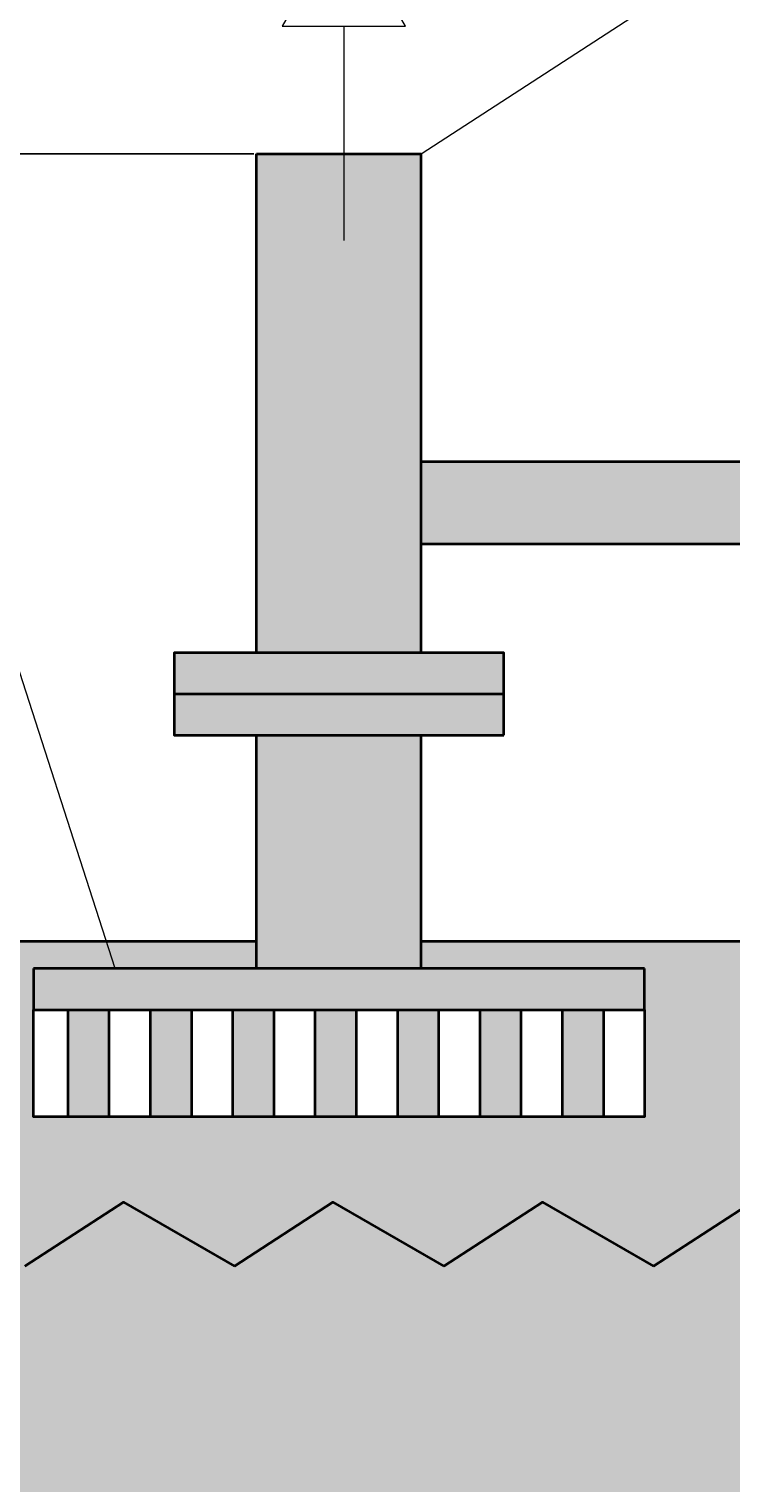
# Model space of a CAD drawing. Units: inches. Extents: x -1 to 292, y -3 to 199.
# Tile 28 of 52: x 106 to 123, y 95 to 130. Entities that reach past the tile are written whole.
import ezdxf

# ---------------------------------------------------------------- set-up
doc = ezdxf.new("R2010")
doc.units = ezdxf.units.IN
doc.header["$MEASUREMENT"] = 0
for name, color, linetype, lineweight in [('M-ANNO-LEAD', 2, 'Continuous', 18), ('M-ANNO-SYMB', 1, 'Continuous', 18), ('M-DIMS', 2, 'Continuous', 18), ('M-EQPM', 7, 'Continuous', 35), ('M-PATT', 8, 'Continuous', 13)]:
    doc.layers.add(name, color=color, linetype=linetype, lineweight=lineweight)
doc.styles.get("Standard").update_dxf_attribs({"font": 'arial.ttf'})
doc.dimstyles.get("Standard").update_dxf_attribs({"dimtxt": 0.18, "dimasz": 0.18, "dimexe": 0.18, "dimexo": 0.0625, "dimgap": 0.09, "dimtad": 0, "dimtih": 1, "dimtoh": 1, "dimdec": 4, "dimzin": 0, "dimdsep": 46, "dimtxsty": 'Standard', "dimcen": 0.09, "dimadec": 0, "dimazin": 0, "dimtfac": 1, "dimtdec": 4, "dimtofl": 0, "dimtmove": 0, "dimatfit": 3, "dimfxl": 1, "dimtolj": 1, "dimtzin": 0, "dimarcsym": 0})

# ---------------------------------------------------------------- blocks, each defined once
blk = doc.blocks.new('ARROW-STEAM-OUT')
blk.add_line((113.608, 129.862), (113.608, 124.666))
blk.add_lwpolyline([(112.108, 129.862), (115.108, 129.862), (113.608, 132.46)], close=True)
blk = doc.blocks.new('*D8')
at = {"layer": 'Defpoints', "color": 0, "transparency": 16777216}
for p in [(-0.662, 126.765), (111.488, 126.765), (69.013, 25.514)]:
    blk.add_point(p, dxfattribs=at)
at = {"layer": 'M-DIMS', "color": 0, "lineweight": -2, "transparency": 16777216}
for p, q in [((111.426, 126.765), (-0.842, 126.765)), ((-0.662, 126.585), (-0.662, 76.321)), ((-0.662, 25.694), (-0.662, 75.958)), ((68.951, 25.514), (-0.842, 25.514))]:
    blk.add_line(p, q, dxfattribs=at)
at = {"layer": 'M-DIMS', "color": 0, "transparency": 16777216}
for points in [[(-0.692, 126.585), (-0.632, 126.585), (-0.662, 126.765)], [(-0.692, 25.694), (-0.632, 25.694), (-0.662, 25.514)]]:
    blk.add_solid(points, dxfattribs=at)
at = {"layer": 'M-DIMS', "color": 0, "transparency": 16777216, "insert": (-0.662, 76.14), "char_height": 0.18, "attachment_point": 5}
blk.add_mtext('\\A1;101.25', dxfattribs=at)
blk = doc.blocks.new('*D9')
at = {"layer": 'Defpoints', "color": 0, "transparency": 16777216}
for p in [(177.053, 174.363), (49.924, 99.774), (177.053, 99.774)]:
    blk.add_point(p, dxfattribs=at)
at = {"layer": 'M-DIMS', "color": 0, "lineweight": -2, "transparency": 16777216}
for p, q in [((49.924, 99.836), (49.924, 174.543)), ((50.104, 174.363), (113.033, 174.363)), ((176.873, 174.363), (113.943, 174.363)), ((177.053, 99.836), (177.053, 174.543))]:
    blk.add_line(p, q, dxfattribs=at)
at = {"layer": 'M-DIMS', "color": 0, "transparency": 16777216}
for points in [[(50.104, 174.393), (50.104, 174.333), (49.924, 174.363)], [(176.873, 174.393), (176.873, 174.333), (177.053, 174.363)]]:
    blk.add_solid(points, dxfattribs=at)
at = {"layer": 'M-DIMS', "color": 0, "transparency": 16777216, "insert": (113.488, 174.363), "char_height": 0.18, "attachment_point": 5}
blk.add_mtext('\\A1;127.13', dxfattribs=at)

msp = doc.modelspace()

# ---------------------------------------------------------------- hatches: boundary and pattern name
at = {"layer": 'M-PATT'}
h = msp.add_hatch(color=256, dxfattribs=at)
h.set_gradient(color1=(0, 127, 0), color2=(0, 127, 0), tint=1, name='CYLINDER')
h.paths.add_polyline_path([(164.5186, 119.2985), (129.9293, 119.2985), (129.9293, 117.2985), (164.1897, 117.2985)])
h.paths.add_polyline_path([(181.5897, 119.2985), (164.5186, 119.2985), (164.1897, 117.2985), (179.5897, 117.2985), (179.5897, 107.8518), (181.5897, 109.1506)])
h.paths.add_polyline_path([(181.5897, 109.1506), (179.5897, 107.8518), (179.5897, 36.2698), (198.4159, 36.2698), (198.4159, 38.2698), (181.5897, 38.2698)])
h.paths.add_polyline_path([(115.4883, 126.765), (111.4883, 126.765), (111.4883, 114.6589), (115.4883, 114.6589)])
h.paths.add_polyline_path([(123.408, 119.2985), (115.4883, 119.2985), (115.4883, 117.2985), (123.408, 117.2985)])
h.paths.add_polyline_path([(115.4883, 112.6589), (111.4883, 112.6589), (111.4883, 106.9941), (115.4883, 106.9941)])
h.paths.add_polyline_path([(120.9032, 106.9941), (106.0735, 106.9941), (106.0735, 105.9941), (120.9032, 105.9941)])
h.paths.add_polyline_path([(236.4209, 117.5104), (234.9209, 117.5104), (234.9209, 97.1861), (236.4209, 97.1861)])
h.paths.add_polyline_path([(236.4209, 126.4904), (234.9209, 126.4904), (234.9209, 118.9331), (236.4209, 118.9331)])
h.paths.add_polyline_path([(244.9552, 125.7269), (242.9552, 125.7269), (242.9552, 116.8562), (244.9552, 116.8562)])
h.paths.add_polyline_path([(244.9552, 115.1721), (242.9552, 115.1721), (242.9552, 109.7385), (244.9552, 109.7385)])
h.paths.add_polyline_path([(248.4468, 109.7385), (239.4637, 109.7385), (239.4637, 109.4289), (248.4468, 109.4289)])
h = msp.add_hatch(color=256, dxfattribs=at)
h.set_gradient(color1=(209, 156, 199), color2=(0, 255, 255), tint=1, name='CYLINDER')
h.paths.add_polyline_path([(117.4883, 114.6589), (111.4883, 114.6589), (109.4883, 114.6589), (109.4883, 113.6589), (117.4883, 113.6589)])
h.paths.add_polyline_path([(117.4883, 113.6589), (109.4883, 113.6589), (109.4883, 112.6589), (115.4883, 112.6589), (117.4883, 112.6589)])
h.paths.add_polyline_path([(107.9079, 105.9941), (106.9079, 105.9941), (106.9079, 103.3981), (107.9079, 103.3981)])
h.paths.add_polyline_path([(109.9079, 105.9941), (108.9079, 105.9941), (108.9079, 103.3981), (109.9079, 103.3981)])
h.paths.add_polyline_path([(111.9079, 105.9941), (110.9079, 105.9941), (110.9079, 103.3981), (111.9079, 103.3981)])
h.paths.add_polyline_path([(113.9079, 105.9941), (112.9079, 105.9941), (112.9079, 103.3981), (113.9079, 103.3981)])
h.paths.add_polyline_path([(115.9079, 105.9941), (114.9079, 105.9941), (114.9079, 103.3981), (115.9079, 103.3981)])
h.paths.add_polyline_path([(117.9079, 105.9941), (116.9079, 105.9941), (116.9079, 103.3981), (117.9079, 103.3981)])
h.paths.add_polyline_path([(119.9079, 105.9941), (118.9079, 105.9941), (118.9079, 103.3981), (119.9079, 103.3981)])
h.paths.add_polyline_path([(241.1492, 109.4289), (240.1492, 109.4289), (240.1492, 107.2081), (241.1492, 107.2081)])
h.paths.add_polyline_path([(243.1492, 109.4289), (242.1492, 109.4289), (242.1492, 107.2081), (243.1492, 107.2081)])
h.paths.add_polyline_path([(245.1492, 109.4289), (244.1492, 109.4289), (244.1492, 107.2081), (245.1492, 107.2081)])
h.paths.add_polyline_path([(247.1492, 109.4289), (246.1492, 109.4289), (246.1492, 107.2081), (247.1492, 107.2081)])
h = msp.add_hatch(color=256, dxfattribs=at)
h.set_gradient(color1=(237, 31, 36), color2=(242, 113, 114), tint=1, name='CYLINDER')
h.paths.add_polyline_path([(106.0735, 105.9941), (106.0735, 106.9941), (108.0603, 106.9941), (107.8488, 107.6501), (57.8007, 107.6501, 0.4142136), (49.9241, 99.7735), (52.3176, 101.3278), (55.0097, 99.7735), (57.4032, 101.3278), (60.0953, 99.7735), (62.4888, 101.3278), (65.1809, 99.7735), (67.5744, 101.3278), (70.2665, 99.7735), (72.66, 101.3278), (75.3521, 99.7735), (77.7456, 101.3278), (80.4377, 99.7735), (82.8312, 101.3278), (85.5233, 99.7735), (87.9168, 101.3278), (90.6089, 99.7735), (93.0024, 101.3278), (95.6945, 99.7735), (98.088, 101.3278), (100.7801, 99.7735), (103.1736, 101.3278), (105.8657, 99.7735), (108.2592, 101.3278), (110.9513, 99.7735), (113.3448, 101.3278), (116.0369, 99.7735), (118.4304, 101.3278), (121.1225, 99.7735), (123.516, 101.3278), (126.2082, 99.7735), (128.6016, 101.3278), (131.2938, 99.7735), (133.6872, 101.3278), (136.3794, 99.7735), (138.7728, 101.3278), (141.465, 99.7735), (143.8584, 101.3278), (146.5506, 99.7735), (148.944, 101.3278), (151.6362, 99.7735), (154.0296, 101.3278), (156.7218, 99.7735), (159.1152, 101.3278), (160.6222, 100.4578), (160.6222, 107.6501), (115.4883, 107.6501), (115.4883, 106.9941), (120.9032, 106.9941), (120.9032, 105.9941), (120.9032, 103.3981), (106.0735, 103.3981)])
h.paths.add_polyline_path([(169.176, 107.6501), (162.1623, 107.6501), (162.1623, 100.004), (164.2008, 101.3278), (166.893, 99.7735), (169.2864, 101.3278), (171.9786, 99.7735), (174.372, 101.3278), (177.0526, 99.7802, 0.4139642)])
h.paths.add_polyline_path([(111.4883, 107.6501), (107.8488, 107.6501), (108.0603, 106.9941), (111.4883, 106.9941)], flags=17)
h.paths.add_polyline_path([(61.6788, 91.897), (57.8007, 91.897, -0.1099266), (54.4604, 92.6403), (43.2011, 92.6403), (23.9502, 84.4688), (23.9502, 58.376), (43.2011, 47.2615), (50.9409, 47.2615, -0.2705926), (57.8007, 51.2672), (61.6788, 51.2672)])
h.paths.add_polyline_path([(73.6788, 91.897), (70.6788, 91.897), (70.6788, 51.2672), (73.6788, 51.2672)])
h.paths.add_polyline_path([(79.6788, 91.897), (76.6788, 91.897), (76.6788, 51.2672), (79.6788, 51.2672)])
h.paths.add_polyline_path([(67.6788, 91.897), (64.6788, 91.897), (64.6788, 51.2672), (67.6788, 51.2672)])
h.paths.add_polyline_path([(101.6788, 91.897), (82.6788, 91.897), (82.6788, 51.2672), (101.6788, 51.2672)])
h.paths.add_polyline_path([(107.6788, 91.897), (104.6788, 91.897), (104.6788, 51.2672), (107.6788, 51.2672)])
h.paths.add_polyline_path([(113.6788, 91.897), (110.6788, 91.897), (110.6788, 51.2672), (113.6788, 51.2672)])
h.paths.add_polyline_path([(119.6788, 91.897), (116.6788, 91.897), (116.6788, 51.2672), (119.6788, 51.2672)])
h.paths.add_polyline_path([(141.6788, 91.897), (122.6788, 91.897), (122.6788, 51.2672), (141.6788, 51.2672)])
h.paths.add_polyline_path([(147.6788, 91.897), (144.6788, 91.897), (144.6788, 51.2672), (147.6788, 51.2672)])
h.paths.add_polyline_path([(153.6788, 91.897), (150.6788, 91.897), (150.6788, 51.2672), (153.6788, 51.2672)])
h.paths.add_polyline_path([(159.6788, 91.897), (156.6788, 91.897), (156.6788, 51.2672), (159.6788, 51.2672)])
h.paths.add_polyline_path([(179.5897, 92.6403), (172.5163, 92.6403, -0.1099266), (169.176, 91.897), (162.6788, 91.897), (162.6788, 51.2672), (169.176, 51.2672, -0.2705926), (176.0358, 47.2615), (179.5897, 47.2615)])
h.paths.add_polyline_path([(203.0265, 84.4688), (183.7755, 92.6403), (181.5897, 92.6403), (181.5897, 47.2615), (183.7755, 47.2615), (203.0265, 58.376)])
h.paths.add_polyline_path([(184.4188, 61.52), (200.7224, 61.52), (200.7224, 77.7532), (184.4188, 77.7532)], flags=24)
h = msp.add_hatch(color=256, dxfattribs=at)
h.set_gradient(color1=(0, 255, 255), color2=(0, 255, 255), tint=1)
h.paths.add_polyline_path([(75.3521, 99.7735), (72.66, 101.3278), (70.2665, 99.7735), (67.5744, 101.3278), (65.1809, 99.7735), (62.4888, 101.3278), (60.0953, 99.7735), (57.4032, 101.3278), (55.0097, 99.7735), (52.3176, 101.3278), (49.9241, 99.7735, 0.4142136), (57.8007, 91.897), (61.6788, 91.897), (61.6788, 51.2672), (57.8007, 51.2672, 0.8088808), (54.5813, 36.2021), (65.0947, 51.2672), (64.6788, 51.2672), (64.6788, 91.897), (67.6788, 91.897), (67.6788, 51.2672), (65.0947, 51.2672), (54.5813, 36.2021, 0.1056561), (57.8007, 35.5141), (169.176, 35.5141, 1), (169.176, 51.2672), (162.6788, 51.2672), (162.6788, 91.897), (169.176, 91.897, 0.4144629), (177.0526, 99.7802), (174.372, 101.3278), (171.9786, 99.7735), (169.2864, 101.3278), (166.893, 99.7735), (164.2008, 101.3278), (162.1623, 100.004), (162.1623, 96.1027), (160.6222, 96.1027), (160.6222, 100.4578), (159.1152, 101.3278), (156.7218, 99.7735), (154.0296, 101.3278), (151.6362, 99.7735), (148.944, 101.3278), (146.5506, 99.7735), (143.8584, 101.3278), (141.465, 99.7735), (138.7728, 101.3278), (136.3794, 99.7735), (133.6872, 101.3278), (131.2938, 99.7735), (128.6016, 101.3278), (126.2082, 99.7735), (123.516, 101.3278), (121.1225, 99.7735), (118.4304, 101.3278), (116.0369, 99.7735), (113.3448, 101.3278), (110.9513, 99.7735), (108.2592, 101.3278), (105.8657, 99.7735), (103.1736, 101.3278), (100.7801, 99.7735), (98.088, 101.3278), (95.6945, 99.7735), (93.0024, 101.3278), (90.6089, 99.7735), (87.9168, 101.3278), (85.5233, 99.7735), (82.8312, 101.3278), (80.4377, 99.7735), (77.7456, 101.3278)])
h.paths.add_polyline_path([(79.6788, 91.897), (79.6788, 51.2672), (76.6788, 51.2672), (76.6788, 91.897)], flags=16)
h.paths.add_polyline_path([(73.6788, 91.897), (73.6788, 51.2672), (70.6788, 51.2672), (70.6788, 91.897)], flags=16)
h.paths.add_polyline_path([(82.6788, 91.897), (101.6788, 91.897), (101.6788, 51.2672), (82.6788, 51.2672)], flags=16)
h.paths.add_polyline_path([(104.6788, 91.897), (107.6788, 91.897), (107.6788, 51.2672), (104.6788, 51.2672)], flags=16)
h.paths.add_polyline_path([(110.6788, 91.897), (113.6788, 91.897), (113.6788, 51.2672), (110.6788, 51.2672)], flags=16)
h.paths.add_polyline_path([(116.6788, 91.897), (119.6788, 91.897), (119.6788, 51.2672), (116.6788, 51.2672)], flags=16)
h.paths.add_polyline_path([(122.6788, 91.897), (141.6788, 91.897), (141.6788, 51.2672), (144.6788, 51.2672), (144.6788, 91.897), (147.6788, 91.897), (147.6788, 51.2672), (122.6788, 51.2672)], flags=16)
h.paths.add_polyline_path([(150.6788, 91.897), (153.6788, 91.897), (153.6788, 51.2672), (150.6788, 51.2672)], flags=16)
h.paths.add_polyline_path([(156.6788, 91.897), (159.6788, 91.897), (159.6788, 51.2672), (156.6788, 51.2672)], flags=16)

# ---------------------------------------------------------------- linework, layer by layer
at = {"layer": 'M-ANNO-LEAD'}
for p, q in [((115.4883, 126.765), (146.4422, 146.8667)), ((108.0603, 106.9941), (99.4422, 133.7141))]:
    msp.add_line(p, q, dxfattribs=at)
at = {"layer": 'M-EQPM'}
for p, q in [((111.4883, 126.765), (115.4883, 126.765)), ((111.4883, 114.6589), (111.4883, 126.765)), ((115.4883, 114.6589), (115.4883, 126.765)), ((109.4883, 113.6589), (117.4883, 113.6589)), ((111.4883, 106.9941), (111.4883, 112.6589)), ((115.4883, 106.9941), (115.4883, 112.6589)), ((120.9032, 106.9941), (106.0735, 106.9941)), ((106.0735, 106.9941), (106.0735, 105.9941)), ((120.9032, 105.9941), (120.9032, 106.9941)), ((106.9079, 105.9941), (106.9079, 103.3981)), ((107.9079, 105.9941), (107.9079, 103.3981)), ((108.9079, 105.9941), (108.9079, 103.3981)), ((109.9079, 105.9941), (109.9079, 103.3981)), ((110.9079, 105.9941), (110.9079, 103.3981)), ((111.9079, 105.9941), (111.9079, 103.3981)), ((112.9079, 105.9941), (112.9079, 103.3981)), ((113.9079, 105.9941), (113.9079, 103.3981)), ((114.9079, 105.9941), (114.9079, 103.3981)), ((115.9079, 105.9941), (115.9079, 103.3981)), ((116.9079, 105.9941), (116.9079, 103.3981)), ((117.9079, 105.9941), (117.9079, 103.3981)), ((118.9079, 105.9941), (118.9079, 103.3981)), ((119.9079, 105.9941), (119.9079, 103.3981))]:
    msp.add_line(p, q, dxfattribs=at)
for points in [[(115.4883, 119.2985), (123.408, 119.2985)], [(115.4883, 117.2985), (123.408, 117.2985)], [(111.4883, 107.6501), (57.8007, 107.6501)], [(160.6222, 107.6501), (115.4883, 107.6501)], [(105.8657, 99.7735), (108.2592, 101.3278), (110.9513, 99.7735)], [(110.9513, 99.7735), (113.3448, 101.3278), (116.0369, 99.7735)], [(116.0369, 99.7735), (118.4304, 101.3278), (121.1225, 99.7735)], [(121.1225, 99.7735), (123.516, 101.3278), (126.2082, 99.7735)]]:
    msp.add_lwpolyline(points, dxfattribs=at)
for points in [[(117.4883, 112.6589), (117.4883, 114.6589), (111.4883, 114.6589), (109.4883, 114.6589), (109.4883, 112.6589), (115.4883, 112.6589)], [(106.0735, 105.9941), (120.9032, 105.9941), (120.9032, 103.3981), (106.0735, 103.3981)]]:
    msp.add_lwpolyline(points, close=True, dxfattribs=at)
msp.add_lwpolyline([(110.9873, 107.6501), (57.8007, 107.6501, 1), (57.8007, 91.897), (61.6788, 91.897)], format="xyb", dxfattribs=at)

# ---------------------------------------------------------------- block references
at = {"layer": 'M-ANNO-SYMB'}
msp.add_blockref('ARROW-STEAM-OUT', (0, 0), dxfattribs=at)

# ---------------------------------------------------------------- dimensions: what is measured, and where the dimension line sits
at = {"layer": 'M-DIMS'}
dim = msp.add_linear_dim(base=(177.0526, 174.3627), p1=(49.9241, 99.7735), p2=(177.0526, 99.7735), dimstyle='Standard', override={"dimdec": 2, "dimlfac": 1, "dimrnd": 0, "dimzin": 0, "dimdsep": 46, "dimlunit": 2}, dxfattribs=at)
dim.commit()
dim.dimension.update_dxf_attribs({"geometry": '*D9', "text_midpoint": (113.4883, 174.3627)})
dim = msp.add_linear_dim(base=(-0.6625, 126.765), p1=(69.013, 25.5141), p2=(111.4883, 126.765), angle=90, dimstyle='Standard', override={"dimdec": 2, "dimlfac": 1, "dimrnd": 0, "dimzin": 0, "dimdsep": 46, "dimlunit": 2}, dxfattribs=at)
dim.commit()
dim.dimension.update_dxf_attribs({"geometry": '*D8', "text_midpoint": (-0.6625, 76.1396)})

doc.saveas('drawing.dxf')
